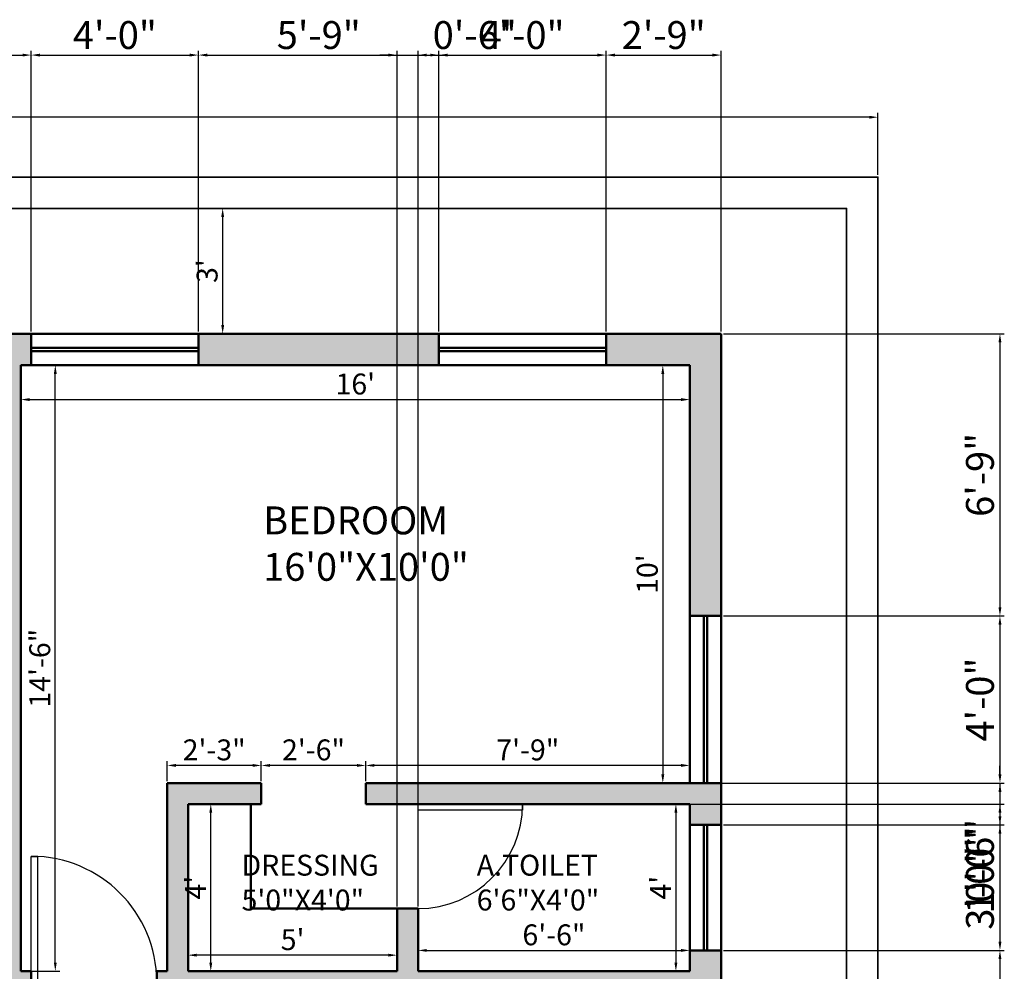
# Model space of a CAD drawing. Units: inches. Extents: x 2442 to 3851, y 589 to 2836.
# Tile 17 of 22: x 2847 to 3130, y 2563 to 2836. Entities that reach past the tile are written whole.
import ezdxf

# ---------------------------------------------------------------- set-up
doc = ezdxf.new("R2010")
doc.units = ezdxf.units.IN
for name, color, linetype, lineweight in [('A-ANNO-DIMS', 2, 'Continuous', 18), ('A-AREA-IDEN', 7, 'Continuous', 18), ('A-DOOR', 4, 'Continuous', 25), ('A-WALL', 7, 'Continuous', 50), ('A-WALL-PATT', 8, 'Continuous', 13), ('C-PROP', 7, 'Continuous', 35)]:
    doc.layers.add(name, color=color, linetype=linetype, lineweight=lineweight)
doc.styles.get("Standard").update_dxf_attribs({"font": 'arial.ttf'})
doc.dimstyles.new('ISO-25', dxfattribs={"dimtxt": 8, "dimasz": 2.5, "dimexe": 1.25, "dimexo": 0.625, "dimtad": 1, "dimlunit": 3, "dimtxsty": 'Standard', "dimcen": 2.5, "dimadec": 0, "dimazin": 0, "dimtfac": 1, "dimtmove": 0, "dimatfit": 3, "dimfxl": 1, "dimarcsym": 0})

# ---------------------------------------------------------------- blocks, each defined once
blk = doc.blocks.new('*U23')
for p, q in [((0, 0), (0, -6)), ((36, 0), (36, -6))]:
    blk.add_line(p, q)
blk.add_lwpolyline([(0, 0), (0, 36), (1.75, 36), (1.75, 0)], close=True)
blk.add_arc((0, 0), 36, 0, 90)
blk = doc.blocks.new('*U24')
for p, q in [((0, 0), (0, -6)), ((30, 0), (30, -6))]:
    blk.add_line(p, q)
blk.add_lwpolyline([(0, 0), (0, 30), (1.75, 30), (1.75, 0)], close=True)
blk.add_arc((0, 0), 30, 0, 90)
blk = doc.blocks.new('*D35')
at = {"layer": 'A-ANNO-DIMS', "color": 0, "lineweight": -2, "transparency": 16777216}
for p, q in [((2493.6, 2791.83), (2493.6, 2809.62)), ((3093.6, 2791.83), (3093.6, 2809.62)), ((3091.1, 2808.37), (2496.1, 2808.37))]:
    blk.add_line(p, q, dxfattribs=at)
at = {"layer": 'A-ANNO-DIMS', "color": 0, "transparency": 16777216}
for points in [[(2496.1, 2808.78), (2496.1, 2807.95), (2493.6, 2808.37)], [(3091.1, 2808.78), (3091.1, 2807.95), (3093.6, 2808.37)]]:
    blk.add_solid(points, dxfattribs=at)
at = {"layer": 'Defpoints', "color": 0, "transparency": 16777216}
for p in [(2493.6, 2808.37), (2493.6, 2791.21), (3093.6, 2791.21)]:
    blk.add_point(p, dxfattribs=at)
at = {"layer": 'A-ANNO-DIMS', "color": 0, "transparency": 16777216, "insert": (2793.6, 2813.08), "char_height": 8, "attachment_point": 5}
blk.add_mtext("50'", dxfattribs=at)
blk = doc.blocks.new('*D43')
at = {"layer": 'A-ANNO-DIMS', "color": 0, "lineweight": -2, "transparency": 16777216}
for p, q in [((2906.15, 2782.21), (2906.78, 2782.21)), ((2905.53, 2748.71), (2905.53, 2779.71)), ((2906.15, 2746.21), (2906.78, 2746.21))]:
    blk.add_line(p, q, dxfattribs=at)
at = {"layer": 'A-ANNO-DIMS', "color": 0, "transparency": 16777216}
for points in [[(2905.11, 2779.71), (2905.95, 2779.71), (2905.53, 2782.21)], [(2905.11, 2748.71), (2905.95, 2748.71), (2905.53, 2746.21)]]:
    blk.add_solid(points, dxfattribs=at)
at = {"layer": 'Defpoints', "color": 0, "transparency": 16777216}
for p in [(2905.53, 2782.21), (2905.53, 2782.21), (2905.53, 2746.21)]:
    blk.add_point(p, dxfattribs=at)
at = {"layer": 'A-ANNO-DIMS', "color": 0, "transparency": 16777216, "insert": (2901.84, 2764.21), "char_height": 6, "attachment_point": 5, "rotation": 90}
blk.add_mtext("3'", dxfattribs=at)
blk = doc.blocks.new('*D46')
at = {"layer": 'A-ANNO-DIMS', "color": 0, "lineweight": -2, "transparency": 16777216}
for p, q in [((2847.6, 2736.58), (2847.6, 2726.07)), ((3039.6, 2736.58), (3039.6, 2726.07)), ((2850.1, 2727.32), (3037.1, 2727.32))]:
    blk.add_line(p, q, dxfattribs=at)
at = {"layer": 'A-ANNO-DIMS', "color": 0, "transparency": 16777216}
for points in [[(2850.1, 2727.74), (2850.1, 2726.91), (2847.6, 2727.32)], [(3037.1, 2727.74), (3037.1, 2726.91), (3039.6, 2727.32)]]:
    blk.add_solid(points, dxfattribs=at)
at = {"layer": 'Defpoints', "color": 0, "transparency": 16777216}
for p in [(2847.6, 2737.21), (3039.6, 2737.21), (3039.6, 2727.32)]:
    blk.add_point(p, dxfattribs=at)
at = {"layer": 'A-ANNO-DIMS', "color": 0, "transparency": 16777216, "insert": (2943.6, 2731.01), "char_height": 6, "attachment_point": 5}
blk.add_mtext("16'", dxfattribs=at)
blk = doc.blocks.new('*D47')
at = {"layer": 'A-ANNO-DIMS', "color": 0, "lineweight": -2, "transparency": 16777216}
for p, q in [((3038.97, 2737.21), (3030.59, 2737.21)), ((3031.84, 2734.71), (3031.84, 2619.71)), ((3038.97, 2617.21), (3030.59, 2617.21))]:
    blk.add_line(p, q, dxfattribs=at)
at = {"layer": 'A-ANNO-DIMS', "color": 0, "transparency": 16777216}
for points in [[(3031.43, 2734.71), (3032.26, 2734.71), (3031.84, 2737.21)], [(3031.43, 2619.71), (3032.26, 2619.71), (3031.84, 2617.21)]]:
    blk.add_solid(points, dxfattribs=at)
at = {"layer": 'Defpoints', "color": 0, "transparency": 16777216}
for p in [(3039.6, 2737.21), (3031.84, 2617.21), (3039.6, 2617.21)]:
    blk.add_point(p, dxfattribs=at)
at = {"layer": 'A-ANNO-DIMS', "color": 0, "transparency": 16777216, "insert": (3028.16, 2677.21), "char_height": 6, "attachment_point": 5, "rotation": 90}
blk.add_mtext("10'", dxfattribs=at)
blk = doc.blocks.new('*D48')
at = {"layer": 'A-ANNO-DIMS', "color": 0, "lineweight": -2, "transparency": 16777216}
for p, q in [((3038.97, 2611.21), (3034.35, 2611.21)), ((3035.6, 2608.71), (3035.6, 2565.71)), ((3038.97, 2563.21), (3034.35, 2563.21))]:
    blk.add_line(p, q, dxfattribs=at)
at = {"layer": 'A-ANNO-DIMS', "color": 0, "transparency": 16777216}
for points in [[(3035.18, 2608.71), (3036.02, 2608.71), (3035.6, 2611.21)], [(3035.18, 2565.71), (3036.02, 2565.71), (3035.6, 2563.21)]]:
    blk.add_solid(points, dxfattribs=at)
at = {"layer": 'Defpoints', "color": 0, "transparency": 16777216}
for p in [(3039.6, 2611.21), (3035.6, 2563.21), (3039.6, 2563.21)]:
    blk.add_point(p, dxfattribs=at)
at = {"layer": 'A-ANNO-DIMS', "color": 0, "transparency": 16777216, "insert": (3031.97, 2587.21), "char_height": 6, "attachment_point": 5, "rotation": 90}
blk.add_mtext("4'", dxfattribs=at)
blk = doc.blocks.new('*D49')
at = {"layer": 'A-ANNO-DIMS', "color": 0, "lineweight": -2, "transparency": 16777216}
for p, q in [((2961.6, 2563.83), (2961.6, 2570.46)), ((2964.1, 2569.21), (3037.1, 2569.21)), ((3039.6, 2563.83), (3039.6, 2570.46))]:
    blk.add_line(p, q, dxfattribs=at)
at = {"layer": 'A-ANNO-DIMS', "color": 0, "transparency": 16777216}
for points in [[(2964.1, 2569.62), (2964.1, 2568.79), (2961.6, 2569.21)], [(3037.1, 2569.62), (3037.1, 2568.79), (3039.6, 2569.21)]]:
    blk.add_solid(points, dxfattribs=at)
at = {"layer": 'Defpoints', "color": 0, "transparency": 16777216}
for p in [(3039.6, 2569.21), (2961.6, 2563.21), (3039.6, 2563.21)]:
    blk.add_point(p, dxfattribs=at)
at = {"layer": 'A-ANNO-DIMS', "color": 0, "transparency": 16777216, "insert": (3000.6, 2572.9), "char_height": 6, "attachment_point": 5}
blk.add_mtext('6\'-6"', dxfattribs=at)
blk = doc.blocks.new('*D50')
at = {"layer": 'A-ANNO-DIMS', "color": 0, "lineweight": -2, "transparency": 16777216}
for p, q in [((2895.6, 2563.83), (2895.6, 2569.09)), ((2955.6, 2563.83), (2955.6, 2569.09)), ((2953.1, 2567.84), (2898.1, 2567.84))]:
    blk.add_line(p, q, dxfattribs=at)
at = {"layer": 'A-ANNO-DIMS', "color": 0, "transparency": 16777216}
for points in [[(2898.1, 2568.26), (2898.1, 2567.43), (2895.6, 2567.84)], [(2953.1, 2568.26), (2953.1, 2567.43), (2955.6, 2567.84)]]:
    blk.add_solid(points, dxfattribs=at)
at = {"layer": 'Defpoints', "color": 0, "transparency": 16777216}
for p in [(2895.6, 2567.84), (2895.6, 2563.21), (2955.6, 2563.21)]:
    blk.add_point(p, dxfattribs=at)
at = {"layer": 'A-ANNO-DIMS', "color": 0, "transparency": 16777216, "insert": (2925.6, 2571.52), "char_height": 6, "attachment_point": 5}
blk.add_mtext("5'", dxfattribs=at)
blk = doc.blocks.new('*D51')
at = {"layer": 'A-ANNO-DIMS', "color": 0, "lineweight": -2, "transparency": 16777216}
for p, q in [((2896.22, 2611.21), (2903.37, 2611.21)), ((2902.12, 2565.71), (2902.12, 2608.71)), ((2896.22, 2563.21), (2903.37, 2563.21))]:
    blk.add_line(p, q, dxfattribs=at)
at = {"layer": 'A-ANNO-DIMS', "color": 0, "transparency": 16777216}
for points in [[(2901.7, 2608.71), (2902.53, 2608.71), (2902.12, 2611.21)], [(2901.7, 2565.71), (2902.53, 2565.71), (2902.12, 2563.21)]]:
    blk.add_solid(points, dxfattribs=at)
at = {"layer": 'Defpoints', "color": 0, "transparency": 16777216}
for p in [(2895.6, 2611.21), (2902.12, 2611.21), (2895.6, 2563.21)]:
    blk.add_point(p, dxfattribs=at)
at = {"layer": 'A-ANNO-DIMS', "color": 0, "transparency": 16777216, "insert": (2898.49, 2587.21), "char_height": 6, "attachment_point": 5, "rotation": 90}
blk.add_mtext("4'", dxfattribs=at)
blk = doc.blocks.new('*D64')
at = {"layer": 'A-ANNO-DIMS', "color": 0, "lineweight": -2, "transparency": 16777216}
for p, q in [((2848.22, 2737.21), (2858.75, 2737.21)), ((2857.5, 2565.71), (2857.5, 2734.71)), ((2848.22, 2563.21), (2858.75, 2563.21))]:
    blk.add_line(p, q, dxfattribs=at)
at = {"layer": 'A-ANNO-DIMS', "color": 0, "transparency": 16777216}
for points in [[(2857.08, 2734.71), (2857.91, 2734.71), (2857.5, 2737.21)], [(2857.08, 2565.71), (2857.91, 2565.71), (2857.5, 2563.21)]]:
    blk.add_solid(points, dxfattribs=at)
at = {"layer": 'Defpoints', "color": 0, "transparency": 16777216}
for p in [(2847.6, 2737.21), (2857.5, 2737.21), (2847.6, 2563.21)]:
    blk.add_point(p, dxfattribs=at)
at = {"layer": 'A-ANNO-DIMS', "color": 0, "transparency": 16777216, "insert": (2853.81, 2650.21), "char_height": 6, "attachment_point": 5, "rotation": 90}
blk.add_mtext('14\'-6"', dxfattribs=at)
blk = doc.blocks.new('*D65')
at = {"layer": 'A-ANNO-DIMS', "color": 0, "lineweight": -2, "transparency": 16777216}
for p, q in [((2946.6, 2617.83), (2946.6, 2623.55)), ((3037.1, 2622.3), (2949.1, 2622.3)), ((3039.6, 2617.83), (3039.6, 2623.55))]:
    blk.add_line(p, q, dxfattribs=at)
at = {"layer": 'A-ANNO-DIMS', "color": 0, "transparency": 16777216}
for points in [[(2949.1, 2622.72), (2949.1, 2621.89), (2946.6, 2622.3)], [(3037.1, 2622.72), (3037.1, 2621.89), (3039.6, 2622.3)]]:
    blk.add_solid(points, dxfattribs=at)
at = {"layer": 'Defpoints', "color": 0, "transparency": 16777216}
for p in [(2946.6, 2622.3), (2946.6, 2617.21), (3039.6, 2617.21)]:
    blk.add_point(p, dxfattribs=at)
at = {"layer": 'A-ANNO-DIMS', "color": 0, "transparency": 16777216, "insert": (2993.1, 2625.99), "char_height": 6, "attachment_point": 5}
blk.add_mtext('7\'-9"', dxfattribs=at)
blk = doc.blocks.new('*D66')
at = {"layer": 'A-ANNO-DIMS', "color": 0, "lineweight": -2, "transparency": 16777216}
for p, q in [((2916.6, 2617.83), (2916.6, 2623.55)), ((2944.1, 2622.3), (2919.1, 2622.3)), ((2946.6, 2617.83), (2946.6, 2623.55))]:
    blk.add_line(p, q, dxfattribs=at)
at = {"layer": 'A-ANNO-DIMS', "color": 0, "transparency": 16777216}
for points in [[(2919.1, 2622.72), (2919.1, 2621.89), (2916.6, 2622.3)], [(2944.1, 2622.72), (2944.1, 2621.89), (2946.6, 2622.3)]]:
    blk.add_solid(points, dxfattribs=at)
at = {"layer": 'Defpoints', "color": 0, "transparency": 16777216}
for p in [(2916.6, 2622.3), (2916.6, 2617.21), (2946.6, 2617.21)]:
    blk.add_point(p, dxfattribs=at)
at = {"layer": 'A-ANNO-DIMS', "color": 0, "transparency": 16777216, "insert": (2931.6, 2625.99), "char_height": 6, "attachment_point": 5}
blk.add_mtext('2\'-6"', dxfattribs=at)
blk = doc.blocks.new('*D67')
at = {"layer": 'A-ANNO-DIMS', "color": 0, "lineweight": -2, "transparency": 16777216}
for p, q in [((2889.6, 2617.83), (2889.6, 2623.55)), ((2914.1, 2622.3), (2892.1, 2622.3)), ((2916.6, 2617.83), (2916.6, 2623.55))]:
    blk.add_line(p, q, dxfattribs=at)
at = {"layer": 'A-ANNO-DIMS', "color": 0, "transparency": 16777216}
for points in [[(2892.1, 2622.72), (2892.1, 2621.89), (2889.6, 2622.3)], [(2914.1, 2622.72), (2914.1, 2621.89), (2916.6, 2622.3)]]:
    blk.add_solid(points, dxfattribs=at)
at = {"layer": 'Defpoints', "color": 0, "transparency": 16777216}
for p in [(2889.6, 2622.3), (2889.6, 2617.21), (2916.6, 2617.21)]:
    blk.add_point(p, dxfattribs=at)
at = {"layer": 'A-ANNO-DIMS', "color": 0, "transparency": 16777216, "insert": (2903.1, 2625.99), "char_height": 6, "attachment_point": 5}
blk.add_mtext('2\'-3"', dxfattribs=at)
blk = doc.blocks.new('*D184')
at = {"layer": 'A-ANNO-DIMS', "color": 0, "lineweight": -2, "transparency": 16777216}
for p, q in [((2796.6, 2746.83), (2796.6, 2827.46)), ((2799.1, 2826.21), (2848.1, 2826.21)), ((2850.6, 2746.83), (2850.6, 2827.46))]:
    blk.add_line(p, q, dxfattribs=at)
at = {"layer": 'A-ANNO-DIMS', "color": 0, "transparency": 16777216}
for points in [[(2799.1, 2826.62), (2799.1, 2825.79), (2796.6, 2826.21)], [(2848.1, 2826.62), (2848.1, 2825.79), (2850.6, 2826.21)]]:
    blk.add_solid(points, dxfattribs=at)
at = {"layer": 'Defpoints', "color": 0, "transparency": 16777216}
for p in [(2850.6, 2826.21), (2796.6, 2746.21), (2850.6, 2746.21)]:
    blk.add_point(p, dxfattribs=at)
at = {"layer": 'A-ANNO-DIMS', "color": 0, "transparency": 16777216, "insert": (2823.6, 2830.92), "char_height": 8, "attachment_point": 5}
blk.add_mtext('4\'-6"', dxfattribs=at)
blk = doc.blocks.new('*D185')
at = {"layer": 'A-ANNO-DIMS', "color": 0, "lineweight": -2, "transparency": 16777216}
for p, q in [((2850.6, 2746.83), (2850.6, 2827.46)), ((2853.1, 2826.21), (2896.1, 2826.21)), ((2898.6, 2746.83), (2898.6, 2827.46))]:
    blk.add_line(p, q, dxfattribs=at)
at = {"layer": 'A-ANNO-DIMS', "color": 0, "transparency": 16777216}
for points in [[(2853.1, 2826.62), (2853.1, 2825.79), (2850.6, 2826.21)], [(2896.1, 2826.62), (2896.1, 2825.79), (2898.6, 2826.21)]]:
    blk.add_solid(points, dxfattribs=at)
at = {"layer": 'Defpoints', "color": 0, "transparency": 16777216}
for p in [(2898.6, 2826.21), (2850.6, 2746.21), (2898.6, 2746.21)]:
    blk.add_point(p, dxfattribs=at)
at = {"layer": 'A-ANNO-DIMS', "color": 0, "transparency": 16777216, "insert": (2874.6, 2830.92), "char_height": 8, "attachment_point": 5}
blk.add_mtext('4\'-0"', dxfattribs=at)
blk = doc.blocks.new('*D186')
at = {"layer": 'A-ANNO-DIMS', "color": 0, "lineweight": -2, "transparency": 16777216}
for p, q in [((2898.6, 2746.83), (2898.6, 2827.46)), ((2901.1, 2826.21), (2965.1, 2826.21)), ((2967.6, 2746.83), (2967.6, 2827.46))]:
    blk.add_line(p, q, dxfattribs=at)
at = {"layer": 'A-ANNO-DIMS', "color": 0, "transparency": 16777216}
for points in [[(2901.1, 2826.62), (2901.1, 2825.79), (2898.6, 2826.21)], [(2965.1, 2826.62), (2965.1, 2825.79), (2967.6, 2826.21)]]:
    blk.add_solid(points, dxfattribs=at)
at = {"layer": 'Defpoints', "color": 0, "transparency": 16777216}
for p in [(2967.6, 2826.21), (2898.6, 2746.21), (2967.6, 2746.21)]:
    blk.add_point(p, dxfattribs=at)
at = {"layer": 'A-ANNO-DIMS', "color": 0, "transparency": 16777216, "insert": (2933.1, 2830.92), "char_height": 8, "attachment_point": 5}
blk.add_mtext('5\'-9"', dxfattribs=at)
blk = doc.blocks.new('*D187')
at = {"layer": 'A-ANNO-DIMS', "color": 0, "lineweight": -2, "transparency": 16777216}
for p, q in [((2967.6, 2746.83), (2967.6, 2827.46)), ((2970.1, 2826.21), (3013.1, 2826.21)), ((3015.6, 2746.83), (3015.6, 2827.46))]:
    blk.add_line(p, q, dxfattribs=at)
at = {"layer": 'A-ANNO-DIMS', "color": 0, "transparency": 16777216}
for points in [[(2970.1, 2826.62), (2970.1, 2825.79), (2967.6, 2826.21)], [(3013.1, 2826.62), (3013.1, 2825.79), (3015.6, 2826.21)]]:
    blk.add_solid(points, dxfattribs=at)
at = {"layer": 'Defpoints', "color": 0, "transparency": 16777216}
for p in [(3015.6, 2826.21), (2967.6, 2746.21), (3015.6, 2746.21)]:
    blk.add_point(p, dxfattribs=at)
at = {"layer": 'A-ANNO-DIMS', "color": 0, "transparency": 16777216, "insert": (2991.6, 2830.92), "char_height": 8, "attachment_point": 5}
blk.add_mtext('4\'-0"', dxfattribs=at)
blk = doc.blocks.new('*D188')
at = {"layer": 'A-ANNO-DIMS', "color": 0, "lineweight": -2, "transparency": 16777216}
for p, q in [((3015.6, 2746.83), (3015.6, 2827.46)), ((3018.1, 2826.21), (3046.1, 2826.21)), ((3048.6, 2746.83), (3048.6, 2827.46))]:
    blk.add_line(p, q, dxfattribs=at)
at = {"layer": 'A-ANNO-DIMS', "color": 0, "transparency": 16777216}
for points in [[(3018.1, 2826.62), (3018.1, 2825.79), (3015.6, 2826.21)], [(3046.1, 2826.62), (3046.1, 2825.79), (3048.6, 2826.21)]]:
    blk.add_solid(points, dxfattribs=at)
at = {"layer": 'Defpoints', "color": 0, "transparency": 16777216}
for p in [(3048.6, 2826.21), (3015.6, 2746.21), (3048.6, 2746.21)]:
    blk.add_point(p, dxfattribs=at)
at = {"layer": 'A-ANNO-DIMS', "color": 0, "transparency": 16777216, "insert": (3032.1, 2830.92), "char_height": 8, "attachment_point": 5}
blk.add_mtext('2\'-9"', dxfattribs=at)
blk = doc.blocks.new('*D189')
at = {"layer": 'A-ANNO-DIMS', "color": 0, "lineweight": -2, "transparency": 16777216}
for p, q in [((3049.22, 2746.21), (3129.85, 2746.21)), ((3128.6, 2743.71), (3128.6, 2667.71)), ((3049.22, 2665.21), (3129.85, 2665.21))]:
    blk.add_line(p, q, dxfattribs=at)
at = {"layer": 'A-ANNO-DIMS', "color": 0, "transparency": 16777216}
for points in [[(3128.18, 2743.71), (3129.02, 2743.71), (3128.6, 2746.21)], [(3128.18, 2667.71), (3129.02, 2667.71), (3128.6, 2665.21)]]:
    blk.add_solid(points, dxfattribs=at)
at = {"layer": 'Defpoints', "color": 0, "transparency": 16777216}
for p in [(3048.6, 2746.21), (3048.6, 2665.21), (3128.6, 2665.21)]:
    blk.add_point(p, dxfattribs=at)
at = {"layer": 'A-ANNO-DIMS', "color": 0, "transparency": 16777216, "insert": (3123.89, 2705.71), "char_height": 8, "attachment_point": 5, "rotation": 90}
blk.add_mtext('6\'-9"', dxfattribs=at)
blk = doc.blocks.new('*D190')
at = {"layer": 'A-ANNO-DIMS', "color": 0, "lineweight": -2, "transparency": 16777216}
for p, q in [((3049.22, 2665.21), (3129.85, 2665.21)), ((3128.6, 2662.71), (3128.6, 2619.71)), ((3049.22, 2617.21), (3129.85, 2617.21))]:
    blk.add_line(p, q, dxfattribs=at)
at = {"layer": 'A-ANNO-DIMS', "color": 0, "transparency": 16777216}
for points in [[(3128.18, 2662.71), (3129.02, 2662.71), (3128.6, 2665.21)], [(3128.18, 2619.71), (3129.02, 2619.71), (3128.6, 2617.21)]]:
    blk.add_solid(points, dxfattribs=at)
at = {"layer": 'Defpoints', "color": 0, "transparency": 16777216}
for p in [(3048.6, 2665.21), (3048.6, 2617.21), (3128.6, 2617.21)]:
    blk.add_point(p, dxfattribs=at)
at = {"layer": 'A-ANNO-DIMS', "color": 0, "transparency": 16777216, "insert": (3123.89, 2641.21), "char_height": 8, "attachment_point": 5, "rotation": 90}
blk.add_mtext('4\'-0"', dxfattribs=at)
blk = doc.blocks.new('*D194')
at = {"layer": 'A-ANNO-DIMS', "color": 0, "lineweight": -2, "transparency": 16777216}
for p, q in [((3049.22, 2617.21), (3129.85, 2617.21)), ((3128.6, 2614.71), (3128.6, 2607.71)), ((3049.22, 2605.21), (3129.85, 2605.21)), ((3128.6, 2605.21), (3128.6, 2580.94))]:
    blk.add_line(p, q, dxfattribs=at)
at = {"layer": 'A-ANNO-DIMS', "color": 0, "transparency": 16777216}
for points in [[(3128.18, 2614.71), (3129.02, 2614.71), (3128.6, 2617.21)], [(3128.18, 2607.71), (3129.02, 2607.71), (3128.6, 2605.21)]]:
    blk.add_solid(points, dxfattribs=at)
at = {"layer": 'Defpoints', "color": 0, "transparency": 16777216}
for p in [(3048.6, 2617.21), (3048.6, 2605.21), (3128.6, 2605.21)]:
    blk.add_point(p, dxfattribs=at)
at = {"layer": 'A-ANNO-DIMS', "color": 0, "transparency": 16777216, "insert": (3123.89, 2591.83), "char_height": 8, "attachment_point": 5, "rotation": 90}
blk.add_mtext('1\'-0"', dxfattribs=at)
blk = doc.blocks.new('*D195')
at = {"layer": 'A-ANNO-DIMS', "color": 0, "lineweight": -2, "transparency": 16777216}
for p, q in [((3049.22, 2605.21), (3129.85, 2605.21)), ((3128.6, 2602.71), (3128.6, 2571.71)), ((3049.22, 2569.21), (3129.85, 2569.21))]:
    blk.add_line(p, q, dxfattribs=at)
at = {"layer": 'A-ANNO-DIMS', "color": 0, "transparency": 16777216}
for points in [[(3128.18, 2602.71), (3129.02, 2602.71), (3128.6, 2605.21)], [(3128.18, 2571.71), (3129.02, 2571.71), (3128.6, 2569.21)]]:
    blk.add_solid(points, dxfattribs=at)
at = {"layer": 'Defpoints', "color": 0, "transparency": 16777216}
for p in [(3048.6, 2605.21), (3048.6, 2569.21), (3128.6, 2569.21)]:
    blk.add_point(p, dxfattribs=at)
at = {"layer": 'A-ANNO-DIMS', "color": 0, "transparency": 16777216, "insert": (3123.89, 2587.21), "char_height": 8, "attachment_point": 5, "rotation": 90}
blk.add_mtext('3\'-0"', dxfattribs=at)
blk = doc.blocks.new('*D196')
at = {"layer": 'A-ANNO-DIMS', "color": 0, "lineweight": -2, "transparency": 16777216}
for p, q in [((3049.22, 2569.21), (3129.85, 2569.21)), ((3128.6, 2566.71), (3128.6, 2550.71)), ((3049.22, 2548.21), (3129.85, 2548.21)), ((3128.6, 2548.21), (3128.6, 2523.94))]:
    blk.add_line(p, q, dxfattribs=at)
at = {"layer": 'A-ANNO-DIMS', "color": 0, "transparency": 16777216}
for points in [[(3128.18, 2566.71), (3129.02, 2566.71), (3128.6, 2569.21)], [(3128.18, 2550.71), (3129.02, 2550.71), (3128.6, 2548.21)]]:
    blk.add_solid(points, dxfattribs=at)
at = {"layer": 'Defpoints', "color": 0, "transparency": 16777216}
for p in [(3048.6, 2569.21), (3048.6, 2548.21), (3128.6, 2548.21)]:
    blk.add_point(p, dxfattribs=at)
at = {"layer": 'A-ANNO-DIMS', "color": 0, "transparency": 16777216, "insert": (3123.89, 2534.83), "char_height": 8, "attachment_point": 5, "rotation": 90}
blk.add_mtext('1\'-9"', dxfattribs=at)
blk = doc.blocks.new('*D216')
at = {"layer": 'A-ANNO-DIMS', "color": 0, "lineweight": -2, "transparency": 16777216}
for p, q in [((2953.1, 2826.21), (2950.6, 2826.21)), ((2955.6, 2581.83), (2955.6, 2827.46)), ((2955.6, 2826.21), (2961.6, 2826.21)), ((2961.6, 2581.83), (2961.6, 2827.46)), ((2964.1, 2826.21), (2989.11, 2826.21))]:
    blk.add_line(p, q, dxfattribs=at)
at = {"layer": 'A-ANNO-DIMS', "color": 0, "transparency": 16777216}
for points in [[(2953.1, 2826.62), (2953.1, 2825.79), (2955.6, 2826.21)], [(2964.1, 2826.62), (2964.1, 2825.79), (2961.6, 2826.21)]]:
    blk.add_solid(points, dxfattribs=at)
at = {"layer": 'Defpoints', "color": 0, "transparency": 16777216}
for p in [(2961.6, 2826.21), (2955.6, 2581.21), (2961.6, 2581.21)]:
    blk.add_point(p, dxfattribs=at)
at = {"layer": 'A-ANNO-DIMS', "color": 0, "transparency": 16777216, "insert": (2977.86, 2830.92), "char_height": 8, "attachment_point": 5}
blk.add_mtext('0\'-6"', dxfattribs=at)
blk = doc.blocks.new('*D217')
at = {"layer": 'A-ANNO-DIMS', "color": 0, "lineweight": -2, "transparency": 16777216}
for p, q in [((3128.6, 2619.71), (3128.6, 2622.21)), ((2947.22, 2617.21), (3129.85, 2617.21)), ((3128.6, 2617.21), (3128.6, 2611.21)), ((2947.22, 2611.21), (3129.85, 2611.21)), ((3128.6, 2608.71), (3128.6, 2583.69))]:
    blk.add_line(p, q, dxfattribs=at)
at = {"layer": 'A-ANNO-DIMS', "color": 0, "transparency": 16777216}
for points in [[(3128.18, 2619.71), (3129.02, 2619.71), (3128.6, 2617.21)], [(3128.18, 2608.71), (3129.02, 2608.71), (3128.6, 2611.21)]]:
    blk.add_solid(points, dxfattribs=at)
at = {"layer": 'Defpoints', "color": 0, "transparency": 16777216}
for p in [(2946.6, 2617.21), (2946.6, 2611.21), (3128.6, 2611.21)]:
    blk.add_point(p, dxfattribs=at)
at = {"layer": 'A-ANNO-DIMS', "color": 0, "transparency": 16777216, "insert": (3123.89, 2594.95), "char_height": 8, "attachment_point": 5, "rotation": 90}
blk.add_mtext('0\'-6"', dxfattribs=at)

msp = doc.modelspace()

# ---------------------------------------------------------------- hatches: boundary and pattern name
at = {"layer": 'A-WALL-PATT'}
h = msp.add_hatch(color=256, dxfattribs=at)
h.dxf.hatch_style = 1
h.paths.add_polyline_path([(2640.599, 2713.208), (2640.599, 2719.208), (2640.599, 2722.208), (2538.599, 2722.208), (2538.599, 2657.708), (2547.599, 2657.708), (2547.599, 2713.208)])
h.paths.add_polyline_path([(2700.599, 2737.208), (2730.599, 2737.208), (2730.599, 2746.208), (2700.599, 2746.208), (2700.599, 2782.208), (2691.599, 2782.208), (2691.599, 2722.208), (2670.599, 2722.208), (2670.599, 2719.208), (2670.599, 2713.208), (2691.599, 2713.208), (2691.599, 2608.208), (2799.599, 2608.208), (2799.599, 2614.208), (2799.599, 2617.208), (2700.599, 2617.208)])
h.paths.add_polyline_path([(2838.599, 2737.208), (2838.599, 2617.208), (2835.599, 2617.208), (2835.599, 2614.208), (2835.599, 2608.208), (2838.599, 2608.208), (2838.599, 2554.208), (2850.599, 2554.208), (2850.599, 2560.208), (2850.599, 2563.208), (2847.599, 2563.208), (2847.599, 2737.208), (2850.599, 2737.208), (2850.599, 2746.208), (2796.599, 2746.208), (2796.599, 2737.208)])
h.paths.add_polyline_path([(2898.599, 2746.208), (2898.599, 2737.208), (2967.599, 2737.208), (2967.599, 2746.208)])
h.paths.add_polyline_path([(3048.599, 2746.208), (3015.599, 2746.208), (3015.599, 2737.208), (3039.599, 2737.208), (3039.599, 2665.208), (3048.599, 2665.208)])
h.paths.add_polyline_path([(3039.599, 2611.208), (3039.599, 2605.208), (3048.599, 2605.208), (3048.599, 2617.208), (2946.599, 2617.208), (2946.599, 2611.208)])
h.paths.add_polyline_path([(2961.599, 2563.208), (2961.599, 2581.208), (2955.599, 2581.208), (2955.599, 2563.208), (2895.599, 2563.208), (2895.599, 2611.208), (2916.599, 2611.208), (2916.599, 2617.208), (2889.599, 2617.208), (2889.599, 2563.208), (2886.599, 2563.208), (2886.599, 2554.208), (2937.599, 2554.208), (2937.599, 2536.208), (2943.599, 2536.208), (2943.599, 2554.208), (3039.599, 2554.208), (3039.599, 2548.208), (3048.599, 2548.208), (3048.599, 2569.208), (3039.599, 2569.208), (3039.599, 2563.208)])
h.paths.add_polyline_path([(2538.599, 2521.208), (2547.599, 2521.208), (2547.599, 2545.208), (2694.599, 2545.208), (2694.599, 2542.208), (2697.599, 2542.208), (2703.599, 2542.208), (2703.599, 2554.208), (2547.599, 2554.208), (2547.599, 2609.708), (2538.599, 2609.708)])
h.paths.add_polyline_path([(2538.599, 2368.208), (2547.599, 2368.208), (2547.599, 2392.208), (2694.599, 2392.208), (2694.599, 2344.208), (2703.599, 2344.208), (2703.599, 2506.208), (2697.599, 2506.208), (2694.599, 2506.208), (2694.599, 2401.208), (2547.599, 2401.208), (2547.599, 2473.208), (2538.599, 2473.208)])
h.paths.add_polyline_path([(2547.599, 2287.208), (2553.599, 2287.208), (2553.599, 2293.208), (2553.599, 2296.208), (2547.599, 2296.208), (2547.599, 2320.208), (2538.599, 2320.208), (2538.599, 2191.208), (2547.599, 2191.208)])
h.paths.add_polyline_path([(2703.599, 2296.208), (2670.599, 2296.208), (2670.599, 2287.208), (2694.599, 2287.208), (2694.599, 2248.208), (2733.599, 2248.208), (2733.599, 2257.208), (2703.599, 2257.208)])
h.paths.add_polyline_path([(2593.599, 2287.208), (2604.599, 2287.208), (2604.599, 2296.208), (2593.599, 2296.208)])
h.paths.add_polyline_path([(2799.599, 2248.208), (2799.599, 2257.208), (2775.599, 2257.208), (2775.599, 2248.208)])
h.paths.add_polyline_path([(2892.599, 2248.208), (2892.599, 2287.208), (2883.599, 2287.208), (2883.599, 2257.208), (2865.599, 2257.208), (2865.599, 2248.208)])
h.paths.add_polyline_path([(2883.599, 2353.208), (2892.599, 2353.208), (2892.599, 2392.208), (3048.599, 2392.208), (3048.599, 2426.708), (3039.599, 2426.708), (3039.599, 2401.208), (2892.599, 2401.208), (2892.599, 2461.208), (2883.599, 2461.208)])
h.paths.add_polyline_path([(3039.599, 2474.708), (3048.599, 2474.708), (3048.599, 2512.208), (3039.599, 2512.208), (3039.599, 2506.208), (2937.599, 2506.208), (2937.599, 2500.208), (3039.599, 2500.208)])

# ---------------------------------------------------------------- linework, layer by layer
at = {"layer": 'A-WALL'}
for p, q in [((2700.599, 2746.208), (3048.599, 2746.208)), ((2850.599, 2737.208), (2850.599, 2746.208)), ((2898.599, 2737.208), (2898.599, 2746.208)), ((2967.599, 2737.208), (2967.599, 2746.208)), ((3015.599, 2737.208), (3015.599, 2746.208)), ((3048.599, 2392.208), (3048.599, 2746.208)), ((2850.599, 2742.208), (2898.599, 2742.208)), ((2850.599, 2741.208), (2898.599, 2741.208)), ((2967.599, 2742.208), (3015.599, 2742.208)), ((2967.599, 2741.208), (3015.599, 2741.208)), ((2847.599, 2563.208), (2847.599, 2737.208)), ((2847.599, 2737.208), (3039.599, 2737.208)), ((3039.599, 2617.208), (3039.599, 2737.208)), ((3039.599, 2665.208), (3048.599, 2665.208)), ((3043.599, 2617.208), (3043.599, 2665.208)), ((3044.599, 2617.208), (3044.599, 2665.208)), ((2889.599, 2563.208), (2889.599, 2617.208)), ((2889.599, 2617.208), (2916.599, 2617.208)), ((2916.599, 2611.208), (2916.599, 2617.208)), ((2946.599, 2611.208), (2946.599, 2617.208)), ((2946.599, 2617.208), (3048.599, 2617.208)), ((2895.599, 2563.208), (2895.599, 2611.208)), ((2895.599, 2611.208), (2916.599, 2611.208)), ((2913.599, 2581.208), (2913.599, 2611.208)), ((2946.599, 2611.208), (3039.599, 2611.208)), ((3039.599, 2563.208), (3039.599, 2611.208)), ((3039.599, 2605.208), (3048.599, 2605.208)), ((3043.599, 2569.208), (3043.599, 2605.208)), ((3044.599, 2569.208), (3044.599, 2605.208)), ((2913.599, 2581.208), (2955.599, 2581.208)), ((2955.599, 2563.208), (2955.599, 2581.208)), ((2955.599, 2581.208), (2961.599, 2581.208)), ((2961.599, 2563.208), (2961.599, 2581.208)), ((3039.599, 2569.208), (3048.599, 2569.208)), ((2847.599, 2563.208), (2850.599, 2563.208)), ((2850.599, 2554.208), (2850.599, 2563.208)), ((2886.599, 2554.208), (2886.599, 2563.208)), ((2886.599, 2563.208), (2889.599, 2563.208)), ((2895.599, 2563.208), (2955.599, 2563.208)), ((2961.599, 2563.208), (3039.599, 2563.208))]:
    msp.add_line(p, q, dxfattribs=at)
at = {"layer": 'C-PROP'}
for points in [[(3066.599, 2191.208), (3093.599, 2191.208), (3093.599, 2791.208), (2493.599, 2791.208), (2493.599, 2191.208), (2738.599, 2191.208)], [(3066.599, 2200.208), (3084.599, 2200.208), (3084.599, 2782.208), (2502.599, 2782.208), (2502.599, 2200.208), (2538.599, 2200.208)]]:
    msp.add_lwpolyline(points, dxfattribs=at)

# ---------------------------------------------------------------- block references
at = {"layer": 'A-DOOR', "rotation": 269.9999999999969}
msp.add_blockref('*U24', (2961.599, 2611.208), dxfattribs=at)
at = {"layer": 'A-DOOR'}
msp.add_blockref('*U23', (2850.599, 2560.208), dxfattribs=at)

# ---------------------------------------------------------------- texts
at = {"layer": 'A-AREA-IDEN', "attachment_point": 1}
for s, insert, char_height in [('{\\fTimes New Roman|b0|i0|c0|p18;BEDROOM\\P16\'0"X10\'0"}', (2917.154, 2696.643), 8), ('{\\fTimes New Roman|b0|i0|c0|p18;DRESSING\\P5\'0"X4\'0"}', (2910.952, 2596.668), 6), ('{\\fTimes New Roman|b0|i0|c0|p18;A.TOILET\\P6\'6"X4\'0"}', (2978.437, 2596.668), 6)]:
    msp.add_mtext_dynamic_manual_height_columns(s, width=110.76054, gutter_width=12.5, heights=[0], dxfattribs=dict(at, insert=insert, char_height=char_height))

# ---------------------------------------------------------------- dimensions: what is measured, and where the dimension line sits
at = {"layer": 'A-ANNO-DIMS'}
for base, p1, p2, override, picture, middle in [((2850.599, 2826.208), (2796.599, 2746.208), (2850.599, 2746.208), {"dimdec": 1, "dimlfac": 1, "dimrnd": 0, "dimzin": 1, "dimdsep": 46, "dimlunit": 4, "dimfrac": 2}, '*D184', (2823.599, 2830.917)), ((2898.599, 2826.208), (2850.599, 2746.208), (2898.599, 2746.208), {"dimdec": 1, "dimlfac": 1, "dimrnd": 0, "dimzin": 1, "dimdsep": 46, "dimlunit": 4, "dimfrac": 2}, '*D185', (2874.599, 2830.917)), ((2967.599, 2826.208), (2898.599, 2746.208), (2967.599, 2746.208), {"dimdec": 1, "dimlfac": 1, "dimrnd": 0, "dimzin": 1, "dimdsep": 46, "dimlunit": 4, "dimfrac": 2}, '*D186', (2933.099, 2830.917)), ((2961.599, 2826.208), (2955.599, 2581.208), (2961.599, 2581.208), {"dimdec": 1, "dimlfac": 1, "dimrnd": 0, "dimzin": 1, "dimdsep": 46, "dimlunit": 4, "dimfrac": 2}, '*D216', (2977.857, 2830.917)), ((3015.599, 2826.208), (2967.599, 2746.208), (3015.599, 2746.208), {"dimdec": 1, "dimlfac": 1, "dimrnd": 0, "dimzin": 1, "dimdsep": 46, "dimlunit": 4, "dimfrac": 2}, '*D187', (2991.599, 2830.917)), ((3048.599, 2826.208), (3015.599, 2746.208), (3048.599, 2746.208), {"dimdec": 1, "dimlfac": 1, "dimrnd": 0, "dimzin": 1, "dimdsep": 46, "dimlunit": 4, "dimfrac": 2}, '*D188', (3032.099, 2830.917)), ((2493.599, 2808.367), (3093.599, 2791.208), (2493.599, 2791.208), {"dimclrd": 0, "dimclre": 0, "dimclrt": 0}, '*D35', (2793.599, 2813.076)), ((3039.599, 2727.324), (2847.599, 2737.208), (3039.599, 2737.208), {"dimtxt": 6, "dimclrd": 0, "dimclre": 0, "dimclrt": 0}, '*D46', (2943.599, 2731.012)), ((2889.599, 2622.302), (2916.599, 2617.208), (2889.599, 2617.208), {"dimtxt": 6, "dimclrd": 0, "dimclre": 0, "dimclrt": 0, "dimtmove": 1}, '*D67', (2903.099, 2625.992)), ((2916.599, 2622.302), (2946.599, 2617.208), (2916.599, 2617.208), {"dimtxt": 6, "dimclrd": 0, "dimclre": 0, "dimclrt": 0, "dimtmove": 1}, '*D66', (2931.599, 2625.99)), ((2946.599, 2622.302), (3039.599, 2617.208), (2946.599, 2617.208), {"dimtxt": 6, "dimclrd": 0, "dimclre": 0, "dimclrt": 0}, '*D65', (2993.099, 2625.99)), ((2895.599, 2567.842), (2955.599, 2563.208), (2895.599, 2563.208), {"dimtxt": 6, "dimclrd": 0, "dimclre": 0, "dimclrt": 0}, '*D50', (2925.599, 2571.518)), ((3039.599, 2569.208), (2961.599, 2563.208), (3039.599, 2563.208), {"dimtxt": 6, "dimclrd": 0, "dimclre": 0, "dimclrt": 0}, '*D49', (3000.599, 2572.896))]:
    dim = msp.add_linear_dim(base=base, p1=p1, p2=p2, dimstyle='ISO-25', override=override, dxfattribs=at)
    dim.commit()
    dim.dimension.update_dxf_attribs({"geometry": picture, "text_midpoint": middle})
for base, p1, p2, override, picture, middle in [((2905.53, 2782.208), (2905.53, 2746.208), (2905.53, 2782.208), {"dimtxt": 6, "dimclrd": 0, "dimclre": 0, "dimclrt": 0}, '*D43', (2901.839, 2764.208)), ((3128.599, 2665.208), (3048.599, 2746.208), (3048.599, 2665.208), {"dimdec": 1, "dimlfac": 1, "dimrnd": 0, "dimzin": 1, "dimdsep": 46, "dimlunit": 4, "dimfrac": 2}, '*D189', (3123.889, 2705.708)), ((2857.496, 2737.208), (2847.599, 2563.208), (2847.599, 2737.208), {"dimtxt": 6, "dimclrd": 0, "dimclre": 0, "dimclrt": 0}, '*D64', (2853.807, 2650.208)), ((3031.844, 2617.208), (3039.599, 2737.208), (3039.599, 2617.208), {"dimtxt": 6, "dimclrd": 0, "dimclre": 0, "dimclrt": 0}, '*D47', (3028.155, 2677.208)), ((3128.599, 2617.208), (3048.599, 2665.208), (3048.599, 2617.208), {"dimdec": 1, "dimlfac": 1, "dimrnd": 0, "dimzin": 1, "dimdsep": 46, "dimlunit": 4, "dimfrac": 2}, '*D190', (3123.889, 2641.208)), ((3128.599, 2611.208), (2946.599, 2617.208), (2946.599, 2611.208), {"dimdec": 1, "dimlfac": 1, "dimrnd": 0, "dimzin": 1, "dimdsep": 46, "dimlunit": 4, "dimfrac": 2}, '*D217', (3123.889, 2594.95)), ((3128.599, 2605.208), (3048.599, 2617.208), (3048.599, 2605.208), {"dimdec": 1, "dimlfac": 1, "dimrnd": 0, "dimzin": 1, "dimdsep": 46, "dimlunit": 4, "dimfrac": 2}, '*D194', (3123.889, 2591.826)), ((2902.117, 2611.208), (2895.599, 2563.208), (2895.599, 2611.208), {"dimtxt": 6, "dimclrd": 0, "dimclre": 0, "dimclrt": 0}, '*D51', (2898.492, 2587.208)), ((3035.599, 2563.208), (3039.599, 2611.208), (3039.599, 2563.208), {"dimtxt": 6, "dimclrd": 0, "dimclre": 0, "dimclrt": 0}, '*D48', (3031.974, 2587.208)), ((3128.599, 2569.208), (3048.599, 2605.208), (3048.599, 2569.208), {"dimdec": 1, "dimlfac": 1, "dimrnd": 0, "dimzin": 1, "dimdsep": 46, "dimlunit": 4, "dimfrac": 2}, '*D195', (3123.886, 2587.208)), ((3128.599, 2548.208), (3048.599, 2569.208), (3048.599, 2548.208), {"dimdec": 1, "dimlfac": 1, "dimrnd": 0, "dimzin": 1, "dimdsep": 46, "dimlunit": 4, "dimfrac": 2}, '*D196', (3123.889, 2534.826))]:
    dim = msp.add_linear_dim(base=base, p1=p1, p2=p2, angle=90, dimstyle='ISO-25', override=override, dxfattribs=at)
    dim.commit()
    dim.dimension.update_dxf_attribs({"geometry": picture, "text_midpoint": middle})

doc.saveas('drawing.dxf')
